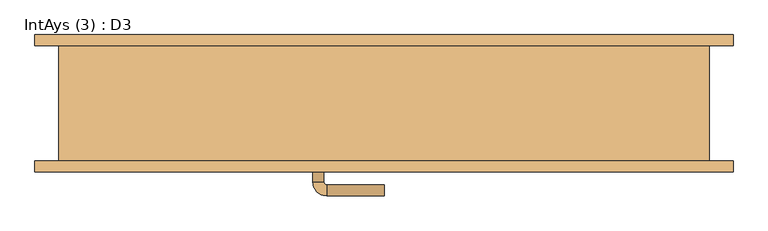
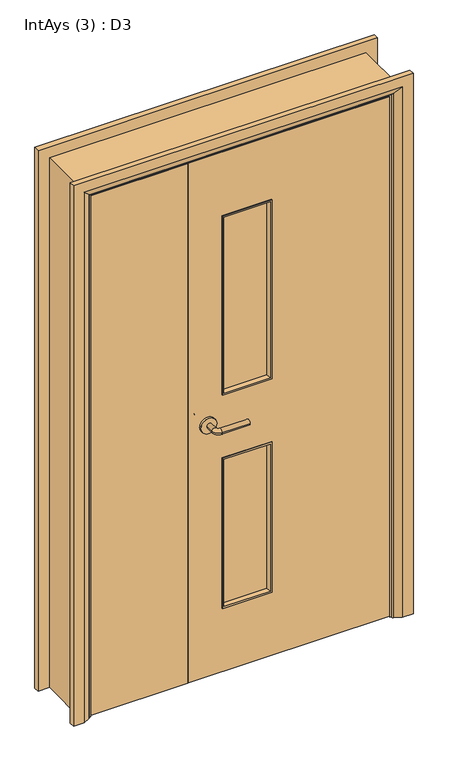
"""IFC4 building model written with IfcOpenShell, lengths in millimetres: door geometry, IntAys (3) : D3."""

from ifc_helpers import new_model, si_unit, point, frame, frame_2d, origin, place, context, project, spatial, polyline, circle_curve, ellipse_curve, trimmed, segment, composite_curve, outline, extrude, faceted_brep, source, transform, mapped, element, save
from ifc_brep_helpers import plane_surface, cylinder_surface, revolved_surface, advanced_brep


def intays_3_d3_2b31a8ce(model_context):
    return source(origin(), model_context, "Body", "SolidModel", [
        advanced_brep(
        [(109.5, -65.0, 1000.0), (129.5, -65.0, 1000.0), (109.5, -35.0, 1000.0), (129.5, -35.0, 1000.0), (134.5, -30.0, 1000.0), (134.5, -10.0, 1000.0), (239.5, -10.0, 1000.0), (239.5, -30.0, 1000.0)],
        [
            (0, 1, circle_curve(frame((119.5, -65.0, 1000.0), z_axis=(0.0, -1.0, 0.0), x_axis=(1.0, 0.0, 0.0)), 10.0)),
            (1, 0, circle_curve(frame((119.5, -65.0, 1000.0), z_axis=(0.0, -1.0, 0.0), x_axis=(1.0, 0.0, 0.0)), 10.0)),
            (0, 2),
            (2, 3, circle_curve(frame((119.5, -35.0, 1000.0), z_axis=(0.0, -1.0, 0.0), x_axis=(1.0, 0.0, 0.0)), 10.0)),
            (3, 1),
            (3, 2, circle_curve(frame((119.5, -35.0, 1000.0), z_axis=(0.0, -1.0, 0.0), x_axis=(1.0, 0.0, 0.0)), 10.0)),
            (4, 3, circle_curve(frame((134.5, -35.0, 1000.0), z_axis=(0.0, 0.0, 1.0), x_axis=(-1.0, 0.0, 0.0)), 5.0)),
            (2, 5, circle_curve(frame((134.5, -35.0, 1000.0), z_axis=(0.0, 0.0, -1.0), x_axis=(-1.0, 0.0, 0.0)), 25.0)),
            (5, 4, circle_curve(frame((134.5, -20.0, 1000.0), z_axis=(-1.0, 0.0, 0.0), x_axis=(0.0, -1.0, 0.0)), 10.0)),
            (4, 5, circle_curve(frame((134.5, -20.0, 1000.0), z_axis=(-1.0, 0.0, 0.0), x_axis=(0.0, -1.0, 0.0)), 10.0)),
            (6, 7, circle_curve(frame((239.5, -20.0, 1000.0), z_axis=(1.0, 0.0, 0.0), x_axis=(0.0, -1.0, 0.0)), 10.0)),
            (7, 6, circle_curve(frame((239.5, -20.0, 1000.0), z_axis=(1.0, 0.0, 0.0), x_axis=(0.0, -1.0, 0.0)), 10.0)),
            (5, 6),
            (7, 4),
        ],
        [
            plane_surface(frame((119.5, -65.0, 1000.0), z_axis=(0.0, -1.0, 0.0), x_axis=(0.0, 0.0, 1.0))),
            cylinder_surface(frame((119.5, -65.0, 1000.0), z_axis=(0.0, -1.0, 0.0), x_axis=(1.0, 0.0, 0.0)), 10.0),
            revolved_surface(trimmed(ellipse_curve(frame((119.5, -35.0, 1000.0), z_axis=(0.0, -1.0, 0.0), x_axis=(1.0, 0.0, 0.0)), 10.0, 10.0), [point((109.5, -35.0, 1000.0))], [point((129.5, -35.0, 1000.0))], True, "CARTESIAN"), (134.5, -35.0, 1000.0), (0.0, 0.0, -1.0)),
            revolved_surface(trimmed(ellipse_curve(frame((119.5, -35.0, 1000.0), z_axis=(0.0, -1.0, 0.0), x_axis=(1.0, 0.0, 0.0)), 10.0, 10.0), [point((129.5, -35.0, 1000.0))], [point((109.5, -35.0, 1000.0))], True, "CARTESIAN"), (134.5, -35.0, 1000.0), (0.0, 0.0, -1.0)),
            plane_surface(frame((239.5, -20.0, 1000.0), z_axis=(1.0, 0.0, 0.0), x_axis=(0.0, 0.0, 1.0))),
            cylinder_surface(frame((134.5, -20.0, 1000.0), z_axis=(-1.0, 0.0, 0.0), x_axis=(0.0, -1.0, 0.0)), 10.0),
        ],
        [
            (0, [[1, 2]]),
            (1, [[-1, 3, 4, 5]]),
            (1, [[-2, -5, 6, -3]]),
            (2, [[7, -4, 8, 9]]),
            (3, [[-8, -6, -7, 10]]),
            (4, [[11, 12]]),
            (5, [[-9, 13, -12, 14]]),
            (5, [[-10, -14, -11, -13]]),
        ],
    ),
        extrude(outline(composite_curve([segment(trimmed(circle_curve(frame_2d((1000.0, 117.0)), 30.0), [point((1000.0, 87.0))], [point((1000.0, 147.0))], False, "CARTESIAN"), True, "CONTINUOUS"), segment(trimmed(circle_curve(frame_2d((1000.0, 117.0)), 30.0), [point((1000.0, 147.0))], [point((1000.0, 87.0))], False, "CARTESIAN"), True, "CONTINUOUS")], self_intersect=False)), frame((0.0, -73.0, 0.0), z_axis=(0.0, 1.0, 0.0), x_axis=(0.0, 0.0, 1.0)), (0.0, 0.0, 1.0), 8.0),
        advanced_brep(
        [(109.5, -113.0, 1000.0), (129.5, -113.0, 1000.0), (129.5, -143.0, 1000.0), (109.5, -143.0, 1000.0), (134.5, -148.0, 1000.0), (134.5, -168.0, 1000.0), (239.5, -168.0, 1000.0), (239.5, -148.0, 1000.0)],
        [
            (0, 1, circle_curve(frame((119.5, -113.0, 1000.0), z_axis=(0.0, 1.0, 0.0), x_axis=(1.0, 0.0, 0.0)), 10.0)),
            (1, 0, circle_curve(frame((119.5, -113.0, 1000.0), z_axis=(0.0, 1.0, 0.0), x_axis=(1.0, 0.0, 0.0)), 10.0)),
            (1, 2),
            (2, 3, circle_curve(frame((119.5, -143.0, 1000.0), z_axis=(0.0, 1.0, 0.0), x_axis=(1.0, 0.0, 0.0)), 10.0)),
            (3, 0),
            (3, 2, circle_curve(frame((119.5, -143.0, 1000.0), z_axis=(0.0, 1.0, 0.0), x_axis=(1.0, 0.0, 0.0)), 10.0)),
            (4, 5, circle_curve(frame((134.5, -158.0, 1000.0), z_axis=(-1.0, 0.0, 0.0), x_axis=(0.0, 1.0, 0.0)), 10.0)),
            (5, 3, circle_curve(frame((134.5, -143.0, 1000.0), z_axis=(0.0, 0.0, -1.0), x_axis=(-1.0, 0.0, 0.0)), 25.0)),
            (2, 4, circle_curve(frame((134.5, -143.0, 1000.0), z_axis=(0.0, 0.0, 1.0), x_axis=(-1.0, 0.0, 0.0)), 5.0)),
            (5, 4, circle_curve(frame((134.5, -158.0, 1000.0), z_axis=(-1.0, 0.0, 0.0), x_axis=(0.0, 1.0, 0.0)), 10.0)),
            (6, 7, circle_curve(frame((239.5, -158.0, 1000.0), z_axis=(1.0, 0.0, 0.0), x_axis=(0.0, 1.0, 0.0)), 10.0)),
            (7, 6, circle_curve(frame((239.5, -158.0, 1000.0), z_axis=(1.0, 0.0, 0.0), x_axis=(0.0, 1.0, 0.0)), 10.0)),
            (4, 7),
            (6, 5),
        ],
        [
            plane_surface(frame((119.5, -113.0, 1000.0), z_axis=(0.0, 1.0, 0.0), x_axis=(0.0, 0.0, 1.0))),
            cylinder_surface(frame((119.5, -113.0, 1000.0), z_axis=(0.0, 1.0, 0.0), x_axis=(1.0, 0.0, 0.0)), 10.0),
            revolved_surface(trimmed(ellipse_curve(frame((119.5, -143.0, 1000.0), z_axis=(0.0, -1.0, 0.0), x_axis=(1.0, 0.0, 0.0)), 10.0, 10.0), [point((109.5, -143.0, 1000.0))], [point((129.5, -143.0, 1000.0))], True, "CARTESIAN"), (134.5, -143.0, 1000.0), (0.0, 0.0, -1.0)),
            revolved_surface(trimmed(ellipse_curve(frame((119.5, -143.0, 1000.0), z_axis=(0.0, -1.0, 0.0), x_axis=(1.0, 0.0, 0.0)), 10.0, 10.0), [point((129.5, -143.0, 1000.0))], [point((109.5, -143.0, 1000.0))], True, "CARTESIAN"), (134.5, -143.0, 1000.0), (0.0, 0.0, -1.0)),
            plane_surface(frame((239.5, -158.0, 1000.0), z_axis=(1.0, 0.0, 0.0), x_axis=(0.0, 0.0, 1.0))),
            cylinder_surface(frame((134.5, -158.0, 1000.0), z_axis=(-1.0, 0.0, 0.0), x_axis=(0.0, 1.0, 0.0)), 10.0),
        ],
        [
            (0, [[1, 2]]),
            (1, [[3, 4, 5, -2]]),
            (1, [[-5, 6, -3, -1]]),
            (2, [[7, 8, -4, 9]]),
            (3, [[10, -9, -6, -8]]),
            (4, [[11, 12]]),
            (5, [[13, -11, 14, -7]]),
            (5, [[-14, -12, -13, -10]]),
        ],
    ),
        extrude(outline(composite_curve([segment(trimmed(circle_curve(frame_2d((1000.0, 117.0)), 30.0), [point((1000.0, 87.0))], [point((1000.0, 147.0))], False, "CARTESIAN"), True, "CONTINUOUS"), segment(trimmed(circle_curve(frame_2d((1000.0, 117.0)), 30.0), [point((1000.0, 147.0))], [point((1000.0, 87.0))], False, "CARTESIAN"), True, "CONTINUOUS")], self_intersect=False)), frame((0.0, -113.0, 0.0), z_axis=(0.0, 1.0, 0.0), x_axis=(0.0, 0.0, 1.0)), (0.0, 0.0, 1.0), 8.0),
        extrude(outline(polyline([(2092.0, -353.0), (0.0, -353.0), (0.0, -321.0), (2060.0, -321.0), (2060.0, 799.0), (0.0, 799.0), (0.0, 831.0), (2092.0, 831.0), (2092.0, -353.0)])), frame((0.0, -105.0, 0.0), z_axis=(0.0, 1.0, 0.0), x_axis=(0.0, 0.0, 1.0)), (0.0, 0.0, 1.0), 210.0),
        faceted_brep([(-302.0, -70.0, 0.0), (-321.0, -70.0, 0.0), (-321.0, -38.0, 0.0), (-302.0, -38.0, 0.0), (-302.0, -38.0, 2041.0), (-302.0, -70.0, 2041.0), (-321.0, -38.0, 2060.0), (-321.0, -70.0, 2060.0), (780.0, -70.0, 0.0), (780.0, -38.0, 0.0), (799.0, -38.0, 0.0), (799.0, -70.0, 0.0), (780.0, -70.0, 2041.0), (799.0, -70.0, 2060.0), (799.0, -38.0, 2060.0), (780.0, -38.0, 2041.0)], [[[0, 1, 2, 3]], [[3, 4, 5, 0]], [[2, 6, 4, 3]], [[1, 7, 6, 2]], [[0, 5, 7, 1]], [[8, 9, 10, 11]], [[12, 8, 11, 13]], [[13, 11, 10, 14]], [[14, 10, 9, 15]], [[15, 9, 8, 12]], [[4, 15, 12, 5]], [[6, 14, 15, 4]], [[7, 13, 14, 6]], [[5, 12, 13, 7]]]),
        advanced_brep(
        [(874.0, -125.0, 0.0), (834.0, -125.0, 0.0), (808.0, -111.0, 0.0), (804.0, -105.0, 0.0), (874.0, -105.0, 0.0), (874.0, -105.0, 2135.0), (874.0, -125.0, 2135.0), (804.0, -105.0, 2065.0), (-326.0, -105.0, 2065.0), (-326.0, -105.0, 0.0), (-396.0, -105.0, 0.0), (-396.0, -105.0, 2135.0), (808.0, -111.0, 2069.0), (834.0, -125.0, 2095.0), (-396.0, -125.0, 2135.0), (-396.0, -125.0, 0.0), (-356.0, -125.0, 0.0), (-356.0, -125.0, 2095.0), (-330.0, -111.0, 0.0), (-330.0, -111.0, 2069.0)],
        [
            (0, 1),
            (1, 2),
            (2, 3, circle_curve(frame((812.0, -104.0, 0.0), z_axis=(0.0, 0.0, -1.0), x_axis=(1.0, 0.0, 0.0)), 8.0622577)),
            (3, 4),
            (4, 0),
            (4, 5),
            (5, 6),
            (6, 0),
            (3, 7),
            (7, 8),
            (8, 9),
            (9, 10),
            (10, 11),
            (11, 5),
            (2, 12),
            (12, 7, ellipse_curve(frame((812.0, -104.0, 2073.0), z_axis=(0.7071067811865475, 0.0, -0.7071067811865475), x_axis=(-0.7071067811865474, 0.0, -0.7071067811865476)), 11.4017543, 8.0622577)),
            (1, 13),
            (13, 12),
            (6, 14),
            (14, 15),
            (15, 16),
            (16, 17),
            (17, 13),
            (10, 15),
            (14, 11),
            (9, 18, circle_curve(frame((-334.0, -104.0, 0.0), z_axis=(0.0, 0.0, -1.0), x_axis=(-1.0, 0.0, 0.0)), 8.0622577)),
            (18, 16),
            (19, 18),
            (8, 19, ellipse_curve(frame((-334.0, -104.0, 2073.0), z_axis=(-0.7071067811865475, 0.0, -0.7071067811865475), x_axis=(-0.7071067811865474, 0.0, 0.7071067811865476)), 11.4017543, 8.0622577)),
            (19, 17),
            (12, 19),
        ],
        [
            plane_surface(frame((804.0, -105.0, 0.0), z_axis=(0.0, 0.0, -1.0), x_axis=(0.0, 1.0, 0.0))),
            plane_surface(frame((874.0, -125.0, 0.0), z_axis=(1.0, 0.0, 0.0), x_axis=(0.0, 0.0, 1.0))),
            plane_surface(frame((874.0, -105.0, 0.0), z_axis=(0.0, 1.0, 0.0), x_axis=(0.0, 0.0, 1.0))),
            cylinder_surface(frame((812.0, -104.0, 0.0), z_axis=(0.0, 0.0, -1.0), x_axis=(1.0, 0.0, 0.0)), 8.0622577),
            plane_surface(frame((808.0, -111.0, 0.0), z_axis=(-0.4740998230350126, -0.8804710999221779, 0.0), x_axis=(0.0, 0.0, 1.0))),
            plane_surface(frame((834.0, -125.0, 0.0), z_axis=(0.0, -1.0, 0.0), x_axis=(0.0, 0.0, 1.0))),
            plane_surface(frame((-396.0, -125.0, 2135.0), z_axis=(-1.0, 0.0, 0.0), x_axis=(0.0, 0.0, -1.0))),
            plane_surface(frame((-326.0, -105.0, 0.0), z_axis=(0.0, 0.0, -1.0), x_axis=(0.0, 1.0, 0.0))),
            cylinder_surface(frame((-334.0, -104.0, 2065.0), z_axis=(0.0, 0.0, 1.0), x_axis=(-1.0, 0.0, 0.0)), 8.0622577),
            plane_surface(frame((-330.0, -111.0, 2069.0), z_axis=(0.4740998230350183, -0.8804710999221749, 0.0), x_axis=(0.0, 0.0, -1.0))),
            plane_surface(frame((874.0, -125.0, 2135.0), z_axis=(0.0, 0.0, 1.0), x_axis=(-1.0, 0.0, 0.0))),
            cylinder_surface(frame((804.0, -104.0, 2073.0), z_axis=(1.0, 0.0, 0.0), x_axis=(0.0, 0.0, 1.0)), 8.0622577),
            plane_surface(frame((808.0, -111.0, 2069.0), z_axis=(0.0, -0.8804710999221763, -0.4740998230350154), x_axis=(-1.0, 0.0, 0.0))),
        ],
        [
            (0, [[1, 2, 3, 4, 5]]),
            (1, [[6, 7, 8, -5]]),
            (2, [[9, 10, 11, 12, 13, 14, -6, -4]]),
            (3, [[15, 16, -9, -3]]),
            (4, [[17, 18, -15, -2]]),
            (5, [[-8, 19, 20, 21, 22, 23, -17, -1]]),
            (6, [[-13, 24, -20, 25]]),
            (7, [[-24, -12, 26, 27, -21]]),
            (8, [[28, -26, -11, 29]]),
            (9, [[-22, -27, -28, 30]]),
            (10, [[-14, -25, -19, -7]]),
            (11, [[31, -29, -10, -16]]),
            (12, [[-23, -30, -31, -18]]),
        ],
    ),
        advanced_brep(
        [(-396.0, 125.0, 0.0), (-356.0, 125.0, 0.0), (-330.0, 111.0, 0.0), (-326.0, 105.0, 0.0), (-396.0, 105.0, 0.0), (-396.0, 105.0, 2135.0), (-396.0, 125.0, 2135.0), (-326.0, 105.0, 2065.0), (804.0, 105.0, 2065.0), (804.0, 105.0, 0.0), (874.0, 105.0, 0.0), (874.0, 105.0, 2135.0), (-330.0, 111.0, 2069.0), (-356.0, 125.0, 2095.0), (874.0, 125.0, 2135.0), (874.0, 125.0, 0.0), (834.0, 125.0, 0.0), (834.0, 125.0, 2095.0), (808.0, 111.0, 0.0), (808.0, 111.0, 2069.0)],
        [
            (0, 1),
            (1, 2),
            (2, 3, circle_curve(frame((-334.0, 104.0, 0.0), z_axis=(0.0, 0.0, -1.0), x_axis=(-1.0, 0.0, 0.0)), 8.0622577)),
            (3, 4),
            (4, 0),
            (4, 5),
            (5, 6),
            (6, 0),
            (3, 7),
            (7, 8),
            (8, 9),
            (9, 10),
            (10, 11),
            (11, 5),
            (2, 12),
            (12, 7, ellipse_curve(frame((-334.0, 104.0, 2073.0), z_axis=(-0.7071067811865475, 0.0, -0.7071067811865475), x_axis=(0.7071067811865474, 0.0, -0.7071067811865476)), 11.4017543, 8.0622577)),
            (1, 13),
            (13, 12),
            (6, 14),
            (14, 15),
            (15, 16),
            (16, 17),
            (17, 13),
            (10, 15),
            (14, 11),
            (9, 18, circle_curve(frame((812.0, 104.0, 0.0), z_axis=(0.0, 0.0, -1.0), x_axis=(1.0, 0.0, 0.0)), 8.0622577)),
            (18, 16),
            (19, 18),
            (8, 19, ellipse_curve(frame((812.0, 104.0, 2073.0), z_axis=(0.7071067811865475, 0.0, -0.7071067811865475), x_axis=(0.7071067811865474, 0.0, 0.7071067811865476)), 11.4017543, 8.0622577)),
            (19, 17),
            (12, 19),
        ],
        [
            plane_surface(frame((-326.0, 105.0, 0.0), z_axis=(0.0, 0.0, -1.0), x_axis=(0.0, 1.0, 0.0))),
            plane_surface(frame((-396.0, 125.0, 0.0), z_axis=(-1.0, 0.0, 0.0), x_axis=(0.0, 0.0, 1.0))),
            plane_surface(frame((-396.0, 105.0, 0.0), z_axis=(0.0, -1.0, 0.0), x_axis=(0.0, 0.0, 1.0))),
            cylinder_surface(frame((-334.0, 104.0, 0.0), z_axis=(0.0, 0.0, -1.0), x_axis=(-1.0, 0.0, 0.0)), 8.0622577),
            plane_surface(frame((-330.0, 111.0, 0.0), z_axis=(0.4740998230350183, 0.8804710999221749, 0.0), x_axis=(0.0, 0.0, 1.0))),
            plane_surface(frame((-356.0, 125.0, 0.0), z_axis=(0.0, 1.0, 0.0), x_axis=(0.0, 0.0, 1.0))),
            plane_surface(frame((874.0, 125.0, 2135.0), z_axis=(1.0, 0.0, 0.0), x_axis=(0.0, 0.0, -1.0))),
            plane_surface(frame((804.0, 105.0, 0.0), z_axis=(0.0, 0.0, -1.0), x_axis=(0.0, 1.0, 0.0))),
            cylinder_surface(frame((812.0, 104.0, 2065.0), z_axis=(0.0, 0.0, 1.0), x_axis=(1.0, 0.0, 0.0)), 8.0622577),
            plane_surface(frame((808.0, 111.0, 2069.0), z_axis=(-0.4740998230350183, 0.8804710999221749, 0.0), x_axis=(0.0, 0.0, -1.0))),
            plane_surface(frame((-396.0, 125.0, 2135.0), z_axis=(0.0, 0.0, 1.0), x_axis=(1.0, 0.0, 0.0))),
            cylinder_surface(frame((-326.0, 104.0, 2073.0), z_axis=(-1.0, 0.0, 0.0), x_axis=(0.0, 0.0, 1.0)), 8.0622577),
            plane_surface(frame((-330.0, 111.0, 2069.0), z_axis=(0.0, 0.8804710999221749, -0.4740998230350183), x_axis=(1.0, 0.0, 0.0))),
        ],
        [
            (0, [[1, 2, 3, 4, 5]]),
            (1, [[6, 7, 8, -5]]),
            (2, [[9, 10, 11, 12, 13, 14, -6, -4]]),
            (3, [[15, 16, -9, -3]]),
            (4, [[17, 18, -15, -2]]),
            (5, [[-8, 19, 20, 21, 22, 23, -17, -1]]),
            (6, [[-13, 24, -20, 25]]),
            (7, [[-24, -12, 26, 27, -21]]),
            (8, [[28, -26, -11, 29]]),
            (9, [[-22, -27, -28, 30]]),
            (10, [[-14, -25, -19, -7]]),
            (11, [[31, -29, -10, -16]]),
            (12, [[-23, -30, -31, -18]]),
        ],
    ),
        extrude(outline(polyline([(5.753223, 796.0), (2057.0, 796.0), (2057.0, 46.0), (5.753223, 46.0), (5.753223, 796.0)]), holes=[polyline([(1807.0, 171.0), (1807.0, 356.0), (1100.0, 356.0), (1100.0, 171.0), (1807.0, 171.0)]), polyline([(850.0, 356.0), (257.0, 356.0), (257.0, 171.0), (850.0, 171.0), (850.0, 356.0)])]), frame((0.0, -105.0, 0.0), z_axis=(0.0, 1.0, 0.0), x_axis=(0.0, 0.0, 1.0)), (0.0, 0.0, 1.0), 32.0),
        extrude(outline(polyline([(43.0, -73.0), (43.0, -105.0), (-318.0, -105.0), (-318.0, -73.0), (43.0, -73.0)])), frame((0.0, 0.0, 5.753223), z_axis=(0.0, 0.0, 1.0), x_axis=(1.0, 0.0, 0.0)), (0.0, 0.0, 1.0), 2051.246777),
        extrude(outline(polyline([(356.0, -83.0), (356.0, -95.0), (171.0, -95.0), (171.0, -83.0), (356.0, -83.0)])), frame((0.0, 0.0, 1100.0), z_axis=(0.0, 0.0, 1.0), x_axis=(1.0, 0.0, 0.0)), (0.0, 0.0, 1.0), 707.0),
        extrude(outline(polyline([(356.0, -83.0), (356.0, -95.0), (171.0, -95.0), (171.0, -83.0), (356.0, -83.0)])), frame((0.0, 0.0, 257.0), z_axis=(0.0, 0.0, 1.0), x_axis=(1.0, 0.0, 0.0)), (0.0, 0.0, 1.0), 593.0),
        faceted_brep([(171.0, -108.0, 1100.0), (171.0, -108.0, 1807.0), (171.0, -95.0, 1807.0), (171.0, -95.0, 1100.0), (183.0, -95.0, 1112.0), (183.0, -95.0, 1795.0), (177.0, -108.0, 1801.0), (177.0, -108.0, 1106.0), (356.0, -108.0, 1807.0), (356.0, -95.0, 1807.0), (344.0, -95.0, 1795.0), (350.0, -108.0, 1801.0), (356.0, -108.0, 1100.0), (356.0, -95.0, 1100.0), (344.0, -95.0, 1112.0), (350.0, -108.0, 1106.0)], [[[0, 1, 2, 3]], [[4, 5, 6, 7]], [[1, 8, 9, 2]], [[5, 10, 11, 6]], [[8, 12, 13, 9]], [[10, 14, 15, 11]], [[3, 2, 9, 13], [5, 4, 14, 10]], [[12, 0, 3, 13]], [[1, 0, 12, 8], [7, 6, 11, 15]], [[14, 4, 7, 15]]]),
        faceted_brep([(356.0, -70.0, 1100.0), (356.0, -70.0, 1807.0), (356.0, -83.0, 1807.0), (356.0, -83.0, 1100.0), (344.0, -83.0, 1112.0), (344.0, -83.0, 1795.0), (350.0, -70.0, 1801.0), (350.0, -70.0, 1106.0), (171.0, -70.0, 1807.0), (171.0, -83.0, 1807.0), (183.0, -83.0, 1795.0), (177.0, -70.0, 1801.0), (171.0, -70.0, 1100.0), (171.0, -83.0, 1100.0), (183.0, -83.0, 1112.0), (177.0, -70.0, 1106.0)], [[[0, 1, 2, 3]], [[4, 5, 6, 7]], [[1, 8, 9, 2]], [[5, 10, 11, 6]], [[8, 12, 13, 9]], [[10, 14, 15, 11]], [[3, 2, 9, 13], [5, 4, 14, 10]], [[12, 0, 3, 13]], [[1, 0, 12, 8], [7, 6, 11, 15]], [[14, 4, 7, 15]]]),
        faceted_brep([(356.0, -70.0, 257.0), (356.0, -70.0, 850.0), (356.0, -83.0, 850.0), (356.0, -83.0, 257.0), (344.0, -83.0, 269.0), (344.0, -83.0, 838.0), (350.0, -70.0, 844.0), (350.0, -70.0, 263.0), (171.0, -70.0, 850.0), (171.0, -83.0, 850.0), (183.0, -83.0, 838.0), (177.0, -70.0, 844.0), (171.0, -70.0, 257.0), (171.0, -83.0, 257.0), (183.0, -83.0, 269.0), (177.0, -70.0, 263.0)], [[[0, 1, 2, 3]], [[4, 5, 6, 7]], [[1, 8, 9, 2]], [[5, 10, 11, 6]], [[8, 12, 13, 9]], [[10, 14, 15, 11]], [[3, 2, 9, 13], [5, 4, 14, 10]], [[12, 0, 3, 13]], [[1, 0, 12, 8], [7, 6, 11, 15]], [[14, 4, 7, 15]]]),
        faceted_brep([(171.0, -108.0, 257.0), (171.0, -108.0, 850.0), (171.0, -95.0, 850.0), (171.0, -95.0, 257.0), (183.0, -95.0, 269.0), (183.0, -95.0, 838.0), (177.0, -108.0, 844.0), (177.0, -108.0, 263.0), (356.0, -108.0, 850.0), (356.0, -95.0, 850.0), (344.0, -95.0, 838.0), (350.0, -108.0, 844.0), (356.0, -108.0, 257.0), (356.0, -95.0, 257.0), (344.0, -95.0, 269.0), (350.0, -108.0, 263.0)], [[[0, 1, 2, 3]], [[4, 5, 6, 7]], [[1, 8, 9, 2]], [[5, 10, 11, 6]], [[8, 12, 13, 9]], [[10, 14, 15, 11]], [[3, 2, 9, 13], [5, 4, 14, 10]], [[12, 0, 3, 13]], [[1, 0, 12, 8], [7, 6, 11, 15]], [[14, 4, 7, 15]]]),
    ])


if __name__ == "__main__":
    model = new_model("IFC4")
    model_context = context("Model", 3, world=origin())
    ifc_project = project(units=[si_unit("LENGTHUNIT", "METRE", prefix="MILLI")], contexts=[model_context])
    site = spatial("IfcSite", under=ifc_project)
    building = spatial("IfcBuilding", under=site)
    placement = place(None, origin())
    intays_3_d3_shape = intays_3_d3_2b31a8ce(model_context)
    element("IfcDoor", 1, ObjectType="IntAys (3) : D3", at=placement, inside=building, context=model_context, shape_type="MappedRepresentation", body=[
        mapped(intays_3_d3_shape, transform((0.0, 0.0, 0.0), x_axis=(1.0, 0.0, 0.0), y_axis=(0.0, 1.0, 0.0), z_axis=(0.0, 0.0, 1.0))),
    ])
    save(model, "model.ifc")

# Revit data of these elements
# Type "IntAys (3) : D3"
#   Type Mark = "57"
#   Type Comments = "Internal Asymmetric"
#   Operation = "DoubleDoorSingleSwing"
#   Keynote = "L20"
#   Description = "Internal Asymmetric Door"
#   VisionPanel Width = 185 mm
#   Thickness = 32 mm
#   Stop Thickness = 19 mm
#   Stop Depth = 32 mm
#   Stile Top of Lock Rail = 1100 mm
#   Stile Top Rail = 250 mm
#   Stile Shutting = 125 mm
#   Stile Lock Rail = 250 mm
#   Stile Intermediate/Frieze = 100 mm
#   Stile Bottom Rail = 250 mm
#   Secondary Panel Width = 361 mm
#   Rough Width = 1200 mm
#   Rough Height = 2100 mm
#   Main Panel Width = 750 mm
#   Handle Z Distance = 1000 mm
#   Handle X Distance = 75 mm
#   Handle Length = 350 mm
#   Frame Thickness = 32 mm
#   Door Panel Width = 750 mm
#   Door Panel Thickness = 32 mm
#   Height = 2100 mm
#   Door Panel Offset = 0 mm
#   Structural Tolerance = 8 mm
#   Tolerance = 3 mm
#   UnderCut = 7 mm
#   Width = 1200 mm
#   Door Panel Height = 2050 mm
#   Architrave Setback = 5 mm
#   Vis - Swing Single = yes
#   Vis - Swing Opposing = no
#   Vis - Swing Double = no
#   Vis - Stops = yes
#   Vis - Ironmongery = yes
#   Material Ironmongery = Door - Handle
#   Material Glass = Door - Glazing
#   Material Frame = Door - Frame/Mullion
#   Material Door = Door - Panel
#   Material Beading = Door - Panel
#   Material Architrave = Door - Architrave
#   Handle Style = element 420585
#   Function = (empty or 0)
#   Wall Closure = (empty or 0)
# Element 1 (IfcDoor, "IntAys (3) : D3")
#   Materials on its faces: "Door - Panel", "Door - Architrave", "Door - Handle", "Door - Frame/Mullion", "Door - Glazing"
# Materials
#   "Door - Handle": colour RGB 0 0 0, transparency 0, Keynote = "P21", Cost = 0, Export to IFC = 0
#   "Door - Glazing": colour RGB 0 0 255, transparency 0.75
#   "Door - Frame/Mullion": class "Wood", colour RGB 212 179 113, transparency 0, Keynote = "L20", Cost = 0, Export to IFC = 0
#   "Door - Panel": class "Wood", colour RGB 210 159 95, transparency 0, Keynote = "L20", Cost = 0, Export to IFC = 0
#   "Door - Architrave": class "Wood", colour RGB 154 90 5, transparency 0, Keynote = "P20", Cost = 0, Export to IFC = 0
